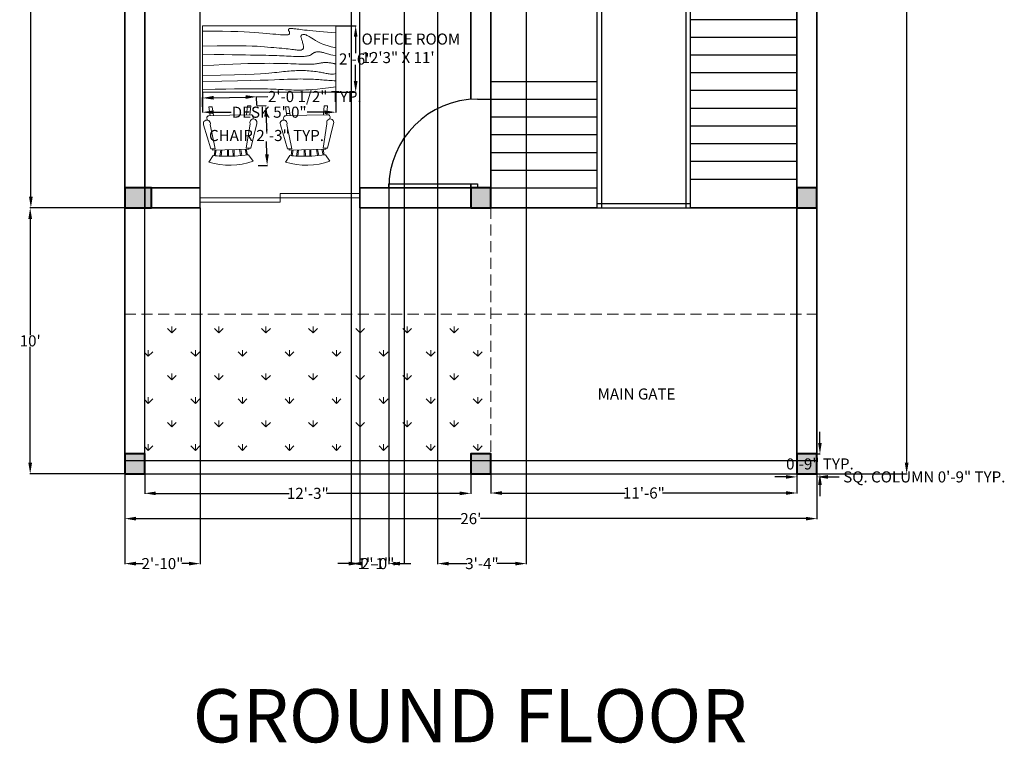
# Model space of a CAD drawing. Units: inches. Extents: x -54 to 881, y -122 to 681.
# Tile 1 of 6: x -47 to 396, y -121 to 205. Entities that reach past the tile are written whole.
import ezdxf

# ---------------------------------------------------------------- set-up
doc = ezdxf.new("R2010")
doc.units = ezdxf.units.IN
doc.header["$MEASUREMENT"] = 0
doc.linetypes.add('DASHED', pattern=[0.75, 0.5, -0.25])
for name, color, linetype, lineweight in [('A-ANNO-DIMS', 2, 'Continuous', 18), ('A-ANNO-TITL', 7, 'Continuous', 35), ('A-DOOR', 3, 'Continuous', 25), ('A-FLOR-OVHD', 8, 'DASHED', 18), ('A-FLOR-STRS', 7, 'Continuous', 25), ('A-FURN', 8, 'Continuous', 18), ('A-GLAZ', 4, 'Continuous', 20), ('A-WALL', 7, 'Continuous', 35), ('A-WALL-SITE', 7, 'Continuous', 30), ('L-PLNT-PATT', 9, 'Continuous', 13)]:
    doc.layers.add(name, color=color, linetype=linetype, lineweight=lineweight)
for name, color, linetype, lineweight, true_color in [('A-ANNO-TEXT', 217, 'Continuous', 18, 0x93278f), ('A-AREA-IDEN', 217, 'Continuous', 18, 0x93278f), ('A-COLS', 240, 'Continuous', 40, 0xed1f24)]:
    doc.layers.add(name, color=color, linetype=linetype, lineweight=lineweight, true_color=true_color)
doc.styles.get("Standard").update_dxf_attribs({"font": 'arial.ttf'})
doc.dimstyles.get("Standard").update_dxf_attribs({"dimtxt": 5, "dimasz": 5, "dimexe": 0.18, "dimexo": 0.0625, "dimgap": 0.09, "dimtad": 0, "dimtih": 1, "dimtoh": 1, "dimdec": 0, "dimzin": 0, "dimdsep": 46, "dimlunit": 3, "dimtxsty": 'Standard', "dimcen": 0.09, "dimadec": 0, "dimazin": 0, "dimtfac": 1, "dimtdec": 0, "dimtofl": 0, "dimtmove": 0, "dimatfit": 3, "dimfxl": 1, "dimtolj": 1, "dimtzin": 0, "dimarcsym": 0})

# ---------------------------------------------------------------- blocks, each defined once
blk = doc.blocks.new('*D2')
at = {"layer": 'A-ANNO-DIMS', "color": 0, "lineweight": -2, "transparency": 16777216}
for p, q in [((-0.06, 624), (-42.51, 624)), ((-42.33, 619), (-42.33, 374.6)), ((-42.33, 125), (-42.33, 369.4)), ((-0.06, 120), (-42.51, 120))]:
    blk.add_line(p, q, dxfattribs=at)
at = {"layer": 'A-ANNO-DIMS', "color": 0, "transparency": 16777216}
for points in [[(-43.17, 619), (-41.5, 619), (-42.33, 624)], [(-43.17, 125), (-41.5, 125), (-42.33, 120)]]:
    blk.add_solid(points, dxfattribs=at)
at = {"layer": 'Defpoints', "color": 0, "transparency": 16777216}
for p in [(0, 624), (-42.33, 120), (0, 120)]:
    blk.add_point(p, dxfattribs=at)
at = {"layer": 'A-ANNO-DIMS', "color": 0, "transparency": 16777216, "insert": (-42.33, 372), "char_height": 5, "attachment_point": 5}
blk.add_mtext("\\A1;42'", dxfattribs=at)
blk = doc.blocks.new('Table - Rectangular Woodgrain 60 x 30 in.')
for p, q in [((0, 0), (0, -30)), ((60, 0), (0, 0)), ((60, -30), (60, 0)), ((0, -30), (60, -30))]:
    blk.add_line(p, q)
for points in [[(0, -2.4), (4.8155, -2.418), (9.0302, -2.4688), (12.709, -2.5477), (15.9167, -2.65), (18.7181, -2.7711), (21.1781, -2.9063), (23.3616, -3.0508), (25.3333, -3.2), (27.1477, -3.3495), (28.8172, -3.4958), (30.3437, -3.636), (31.7291, -3.7667), (32.9756, -3.8849), (34.0849, -3.9875), (35.059, -4.0714), (35.9, -4.1334), (36.6114, -4.1711), (37.2041, -4.1854), (37.6906, -4.1779), (38.0833, -4.15), (38.3948, -4.1034), (38.6375, -4.0396), (38.8239, -3.9602), (38.9666, -3.8667), (39.0764, -3.7608), (39.1573, -3.6448), (39.2116, -3.521), (39.2416, -3.3917), (39.2498, -3.2593), (39.2385, -3.1261), (39.21, -2.9944), (39.1666, -2.8667), (39.111, -2.7447), (39.0468, -2.6281), (38.978, -2.5163), (38.9083, -2.4083), (38.8418, -2.3035), (38.7823, -2.201), (38.7337, -2.1001), (38.7, -2), (38.6844, -1.9003), (38.6875, -1.8021), (38.7094, -1.707), (38.75, -1.6167), (38.8094, -1.5326), (38.8875, -1.4563), (38.9844, -1.3893), (39.1, -1.3333), (39.2351, -1.2896), (39.3937, -1.2583), (39.5804, -1.2396), (39.8, -1.2333), (40.057, -1.2396), (40.3562, -1.2583), (40.7023, -1.2896), (41.1, -1.3333), (41.5547, -1.3895), (42.0755, -1.4573), (42.6721, -1.5361), (43.3542, -1.625), (44.1316, -1.7233), (45.014, -1.8302), (46.0114, -1.9449), (47.1333, -2.0667), (48.3862, -2.1947), (49.7625, -2.3281), (51.2513, -2.4663), (52.8416, -2.6083), (54.5226, -2.7535), (56.2833, -2.9011), (58.1127, -3.0501), (60, -3.2)], [(0, -9.2), (6.5759, -9.0858), (11.9385, -9.0365), (16.2527, -9.0418), (19.6833, -9.0917), (22.3952, -9.1759), (24.5531, -9.2844), (26.322, -9.4069), (27.8666, -9.5333), (29.3241, -9.6553), (30.7203, -9.7719), (32.0532, -9.8837), (33.3208, -9.9917), (34.5213, -10.0965), (35.6526, -10.199), (36.7128, -10.2999), (37.7, -10.4), (38.6129, -10.4996), (39.4531, -10.5969), (40.223, -10.6895), (40.925, -10.775), (41.5613, -10.8512), (42.1344, -10.9156), (42.6465, -10.966), (43.1, -11), (43.4976, -11.0158), (43.8437, -11.0136), (44.143, -10.9942), (44.4, -10.9583), (44.6195, -10.9069), (44.8062, -10.8406), (44.9648, -10.7603), (45.1, -10.6667), (45.2155, -10.5598), (45.3114, -10.4365), (45.3871, -10.2929), (45.4416, -10.125), (45.4743, -9.929), (45.4844, -9.7011), (45.4709, -9.4371), (45.4333, -9.1333), (45.3716, -8.7883), (45.2896, -8.4104), (45.1919, -8.0107), (45.0833, -7.6), (44.9685, -7.1893), (44.8521, -6.7896), (44.7388, -6.4117), (44.6333, -6.0667), (44.54, -5.7628), (44.4614, -5.4979), (44.4001, -5.2675), (44.3583, -5.0667), (44.3384, -4.8909), (44.3427, -4.7354), (44.3736, -4.5956), (44.4333, -4.4667), (44.5236, -4.3453), (44.6427, -4.2333), (44.7884, -4.1339), (44.9583, -4.05), (45.1501, -3.9849), (45.3614, -3.9417), (45.59, -3.9234), (45.8333, -3.9333), (46.0915, -3.9749), (46.3734, -4.0531), (46.6906, -4.1736), (47.0542, -4.3417), (47.4756, -4.5629), (47.9661, -4.8427), (48.5372, -5.1866), (49.2, -5.6), (49.9676, -6.0844), (50.8594, -6.625), (51.8965, -7.2031), (53.1, -7.8), (54.491, -8.3969), (56.0906, -8.975), (57.9199, -9.5156), (60, -10)], [(0, -12.8), (5.1847, -12.9322), (9.6213, -13.0323), (13.3963, -13.1059), (16.5958, -13.1583), (19.3063, -13.1952), (21.614, -13.2219), (23.6054, -13.2439), (25.3666, -13.2667), (26.9728, -13.2947), (28.4531, -13.3281), (29.8256, -13.3663), (31.1083, -13.4083), (32.3191, -13.4535), (33.476, -13.501), (34.597, -13.5501), (35.7, -13.6), (36.7984, -13.6497), (37.8875, -13.6979), (38.9578, -13.743), (40, -13.7833), (41.0047, -13.8174), (41.9625, -13.8438), (42.864, -13.8607), (43.7, -13.8667), (44.4631, -13.8604), (45.1552, -13.8417), (45.7801, -13.8104), (46.3416, -13.7667), (46.8439, -13.7104), (47.2906, -13.6417), (47.6858, -13.5604), (48.0333, -13.4667), (48.3375, -13.3608), (48.6042, -13.2448), (48.8396, -13.121), (49.05, -12.9917), (49.2417, -12.8593), (49.4208, -12.7261), (49.5937, -12.5944), (49.7667, -12.4667), (49.9452, -12.3451), (50.1323, -12.2313), (50.3303, -12.1268), (50.5416, -12.0333), (50.7686, -11.9524), (51.0135, -11.8854), (51.2788, -11.8341), (51.5666, -11.8), (51.8785, -11.7843), (52.2116, -11.7865), (52.562, -11.8059), (52.926, -11.8417), (53.2998, -11.8931), (53.6795, -11.9594), (54.0614, -12.0397), (54.4416, -12.1333), (54.8223, -12.2401), (55.2293, -12.3625), (55.6942, -12.5037), (56.2489, -12.6667), (56.9251, -12.8547), (57.7545, -13.0708), (58.7689, -13.3182), (60, -13.6)], [(0, -18), (5.124, -17.7273), (9.6609, -17.5057), (13.6705, -17.3303), (17.2125, -17.1958), (20.3467, -17.0973), (23.1328, -17.0297), (25.6307, -16.9878), (27.9, -16.9667), (29.9928, -16.9617), (31.9302, -16.9703), (33.7254, -16.9907), (35.3917, -17.0208), (36.9423, -17.0588), (38.3906, -17.1026), (39.7499, -17.1503), (41.0333, -17.2), (42.2519, -17.2496), (43.4073, -17.2969), (44.4986, -17.3395), (45.525, -17.375), (46.4858, -17.4012), (47.3802, -17.4156), (48.2074, -17.416), (48.9667, -17.4), (49.6583, -17.3662), (50.2872, -17.3167), (50.8595, -17.2547), (51.3812, -17.1833), (51.8584, -17.1057), (52.2971, -17.025), (52.7034, -16.9443), (53.0833, -16.8667), (53.443, -16.7951), (53.789, -16.7313), (54.128, -16.6768), (54.4666, -16.6334), (54.8115, -16.6024), (55.1693, -16.5854), (55.5465, -16.5841), (55.95, -16.6), (56.3828, -16.6337), (56.8346, -16.6823), (57.2915, -16.7418), (57.7396, -16.8084), (58.165, -16.878), (58.5539, -16.9469), (58.8924, -17.0111), (59.1666, -17.0667), (59.3679, -17.1107), (59.5078, -17.1438), (59.6032, -17.1675), (59.6708, -17.1833), (59.7275, -17.193), (59.7901, -17.1979), (59.8753, -17.1998), (60, -17.2)], [(0, -22.4), (8.0098, -22.2501), (14.4094, -22.1011), (19.4168, -21.9535), (23.25, -21.8083), (26.1269, -21.6663), (28.2656, -21.5281), (29.884, -21.3947), (31.2, -21.2667), (32.3967, -21.1448), (33.5172, -21.0292), (34.5697, -20.9198), (35.5625, -20.8167), (36.5037, -20.7198), (37.4015, -20.6292), (38.2642, -20.5448), (39.1, -20.4667), (39.9164, -20.3951), (40.7187, -20.3313), (41.5117, -20.2768), (42.3, -20.2333), (43.0883, -20.2024), (43.8812, -20.1854), (44.6836, -20.1841), (45.5, -20.2), (46.3328, -20.234), (47.1747, -20.2844), (48.0163, -20.3488), (48.8479, -20.425), (49.66, -20.5106), (50.4429, -20.6031), (51.1872, -20.7004), (51.8833, -20.8), (52.5246, -20.8999), (53.1166, -20.9995), (53.6681, -21.0983), (54.1875, -21.1958), (54.6834, -21.2919), (55.1646, -21.3859), (55.6394, -21.4777), (56.1167, -21.5667), (56.6028, -21.6515), (57.0961, -21.7266), (57.5929, -21.7852), (58.0896, -21.8208), (58.5823, -21.8268), (59.0674, -21.7964), (59.5412, -21.723), (60, -21.6)], [(0, -25.2), (8.6355, -25.0504), (15.7026, -24.9031), (21.4049, -24.7606), (25.9458, -24.625), (29.529, -24.4988), (32.3578, -24.3844), (34.6359, -24.284), (36.5667, -24.2), (38.3213, -24.1341), (39.9417, -24.0854), (41.437, -24.0523), (42.8167, -24.0333), (44.0901, -24.0268), (45.2667, -24.0313), (46.3557, -24.0451), (47.3667, -24.0667), (48.309, -24.0947), (49.1928, -24.1287), (50.0284, -24.168), (50.826, -24.2125), (51.5959, -24.2617), (52.3483, -24.3151), (53.0935, -24.3725), (53.8417, -24.4334), (54.6009, -24.497), (55.3699, -24.561), (56.1454, -24.6226), (56.9239, -24.6792), (57.7021, -24.7279), (58.4764, -24.7662), (59.2435, -24.7911), (60, -24.8)], [(0, -28.8), (5.6867, -28.6681), (10.45, -28.5698), (14.407, -28.5012), (17.675, -28.4584), (20.3711, -28.4374), (22.6125, -28.4344), (24.5164, -28.4455), (26.2, -28.4667), (27.762, -28.4947), (29.2276, -28.5281), (30.6033, -28.5663), (31.8958, -28.6084), (33.1118, -28.6535), (34.2578, -28.7011), (35.3405, -28.7501), (36.3666, -28.8), (37.3443, -28.8497), (38.288, -28.8974), (39.2137, -28.9412), (40.1375, -28.9792), (41.0753, -29.0093), (42.0432, -29.0297), (43.0572, -29.0384), (44.1333, -29.0333), (45.2936, -29.0114), (46.5843, -28.9641), (48.0579, -28.8816), (49.7666, -28.7542), (51.7629, -28.5721), (54.0989, -28.3255), (56.8272, -28.0048), (60, -27.6)]]:
    blk.add_lwpolyline(points)
blk = doc.blocks.new('Chair - Rocking')
for p, q in [((-8, -4.5), (-10, -1.5)), ((-6.5, -7), (-7.02225, -4.43)), ((-4.5, -7), (-4.96674, -4.19951)), ((-4, -7), (-4.40532, -4.16272)), ((-1.5, -4.05012), (-1.5, -7)), ((-1, -7), (-1, -4.05012)), ((1, -7), (1, -4.04655)), ((1.5, -4.05012), (1.5, -7)), ((4, -7), (4.40187, -4.18694)), ((4.5, -7), (4.96761, -4.19437)), ((6.5, -7), (7, -4.4057)), ((8, -4.5), (10, -1.5)), ((-9, -7.5), (-12, -18.49999)), ((-7, -7.5), (-9, -7.5)), ((-9, -18.49999), (-7, -7.5)), ((-8.23428, -6.99939), (-8.3093, -7.47958)), ((-8.23041, -7), (8.23915, -7)), ((-7.5, -4.5), (-7, -7)), ((7.5, -4.5), (7, -7)), ((7, -7.5), (9, -7.5)), ((9, -18.49999), (7, -7.5)), ((8.31071, -7.48854), (8.23449, -7.00073)), ((9, -7.5), (12, -18.49999)), ((-10.36644, -20.64523), (-10.5, -21.49999)), ((10.5, -21.49999), (10.3575, -20.58798)), ((-9, -22.49999), (-9.5, -26.49999)), ((0, -22.49999), (-9.5, -22.49999)), ((-9.5, -26.49999), (-8, -26.49999)), ((-8, -26.49999), (-7.5, -22.49999)), ((0, -22.49999), (9.5, -22.49999)), ((8, -26.49999), (7.5, -22.49999)), ((9.5, -26.49999), (8, -26.49999)), ((9, -22.49999), (9.5, -26.49999))]:
    blk.add_line(p, q)
for centre, radius, start, end in [((0, -34.08333), 34.08333, 72.93847, 107.0615), ((0, -68.25004), 64.25, 93.92211, 97.15267), ((0, -68.25004), 64.25, 82.84733, 93.92211), ((-10.5, -18.99999), 1.58114, 161.5651, 18.43495), ((-9.5, -21.49999), 1, 180, 270), ((10.5, -18.99999), 1.58114, 161.5651, 18.43495), ((9.5, -21.49999), 1, 270, 0)]:
    blk.add_arc(centre, radius, start, end)
blk = doc.blocks.new('*U12')
for p, q in [((0, 0), (0, -6)), ((40, 0), (40, -6))]:
    blk.add_line(p, q)
blk.add_lwpolyline([(0, 0), (0, 40), (1.75, 40), (1.75, 0)], close=True)
blk.add_arc((0, 0), 40, 0, 90)
blk = doc.blocks.new('*D17')
at = {"layer": 'A-ANNO-DIMS', "color": 0, "lineweight": -2, "transparency": 16777216}
for p, q in [((-0.06, 120), (-42.81, 120)), ((-42.63, 115), (-42.63, 62.64)), ((-42.63, 5), (-42.63, 57.36)), ((-0.06, 0), (-42.81, 0))]:
    blk.add_line(p, q, dxfattribs=at)
at = {"layer": 'A-ANNO-DIMS', "color": 0, "transparency": 16777216}
for points in [[(-43.46, 115), (-41.8, 115), (-42.63, 120)], [(-43.46, 5), (-41.8, 5), (-42.63, 0)]]:
    blk.add_solid(points, dxfattribs=at)
at = {"layer": 'Defpoints', "color": 0, "transparency": 16777216}
for p in [(0, 120), (0, 0), (-42.63, 0)]:
    blk.add_point(p, dxfattribs=at)
at = {"layer": 'A-ANNO-DIMS', "color": 0, "transparency": 16777216, "insert": (-42.63, 60), "char_height": 5, "attachment_point": 5}
blk.add_mtext("\\A1;10'", dxfattribs=at)
blk = doc.blocks.new('*D18')
at = {"layer": 'A-ANNO-DIMS', "color": 0, "lineweight": -2, "transparency": 16777216}
for p, q in [((9, -0.06), (9, -8.94)), ((156, -0.06), (156, -8.94)), ((14, -8.76), (74.06, -8.76)), ((151, -8.76), (90.94, -8.76))]:
    blk.add_line(p, q, dxfattribs=at)
at = {"layer": 'A-ANNO-DIMS', "color": 0, "transparency": 16777216}
for points in [[(14, -7.93), (14, -9.59), (9, -8.76)], [(151, -7.93), (151, -9.59), (156, -8.76)]]:
    blk.add_solid(points, dxfattribs=at)
at = {"layer": 'Defpoints', "color": 0, "transparency": 16777216}
for p in [(9, 0), (156, 0), (156, -8.76)]:
    blk.add_point(p, dxfattribs=at)
at = {"layer": 'A-ANNO-DIMS', "color": 0, "transparency": 16777216, "insert": (82.5, -8.76), "char_height": 5, "attachment_point": 5}
blk.add_mtext('\\A1;12\'-3"', dxfattribs=at)
blk = doc.blocks.new('*D19')
at = {"layer": 'A-ANNO-DIMS', "color": 0, "lineweight": -2, "transparency": 16777216}
for p, q in [((165, -0.06), (165, -8.79)), ((303, -0.06), (303, -8.79)), ((170, -8.61), (225.56, -8.61)), ((298, -8.61), (242.44, -8.61))]:
    blk.add_line(p, q, dxfattribs=at)
at = {"layer": 'A-ANNO-DIMS', "color": 0, "transparency": 16777216}
for points in [[(170, -7.78), (170, -9.45), (165, -8.61)], [(298, -7.78), (298, -9.45), (303, -8.61)]]:
    blk.add_solid(points, dxfattribs=at)
at = {"layer": 'Defpoints', "color": 0, "transparency": 16777216}
for p in [(165, 0), (303, 0), (303, -8.61)]:
    blk.add_point(p, dxfattribs=at)
at = {"layer": 'A-ANNO-DIMS', "color": 0, "transparency": 16777216, "insert": (234, -8.61), "char_height": 5, "attachment_point": 5}
blk.add_mtext('\\A1;11\'-6"', dxfattribs=at)
blk = doc.blocks.new('*D20')
at = {"layer": 'A-ANNO-DIMS', "color": 0, "lineweight": -2, "transparency": 16777216}
for p, q in [((0, -0.06), (0, -20.34)), ((312, -0.06), (312, -20.34)), ((5, -20.16), (151.62, -20.16)), ((307, -20.16), (160.38, -20.16))]:
    blk.add_line(p, q, dxfattribs=at)
at = {"layer": 'A-ANNO-DIMS', "color": 0, "transparency": 16777216}
for points in [[(5, -19.33), (5, -20.99), (0, -20.16)], [(307, -19.33), (307, -20.99), (312, -20.16)]]:
    blk.add_solid(points, dxfattribs=at)
at = {"layer": 'Defpoints', "color": 0, "transparency": 16777216}
for p in [(0, 0), (312, 0), (312, -20.16)]:
    blk.add_point(p, dxfattribs=at)
at = {"layer": 'A-ANNO-DIMS', "color": 0, "transparency": 16777216, "insert": (156, -20.16), "char_height": 5, "attachment_point": 5}
blk.add_mtext("\\A1;26'", dxfattribs=at)
blk = doc.blocks.new('STAIR-RETURN-FLIGHT')
for p, q in [((48, 93), (48, 141)), ((56.4, 93), (56.4, 141)), ((64.8, 93), (64.8, 141)), ((73.2, 93), (73.2, 141)), ((81.6, 93), (81.6, 141)), ((90, 93), (90, 141)), ((48, 0), (48, 93)), ((48, 93), (90, 93)), ((48, 91), (90, 91)), ((50, 0), (50, 93)), ((88, 0), (88, 93)), ((90, 0), (90, 93)), ((90, 93), (138, 93)), ((90, 85), (138, 85)), ((90, 77), (138, 77)), ((90, 69), (138, 69)), ((90, 61), (138, 61)), ((0, 57), (48, 57)), ((0, 49), (48, 49)), ((90, 53), (138, 53)), ((90, 45), (138, 45)), ((0, 41), (48, 41)), ((90, 37), (138, 37)), ((0, 33), (48, 33)), ((90, 29), (138, 29)), ((0, 25), (48, 25)), ((90, 21), (138, 21)), ((0, 17), (48, 17)), ((0, 9), (48, 9)), ((90, 13), (138, 13)), ((48, 2), (90, 2)), ((48, 0), (90, 0))]:
    blk.add_line(p, q)
blk = doc.blocks.new('COL-9X12')
h = blk.add_hatch(color=256)
h.dxf.hatch_style = 1
h.paths.add_polyline_path([(9, 12), (0, 12), (0, 0), (9, 0)])
blk.add_lwpolyline([(0, 0), (9, 0), (9, 12), (0, 12)], close=True)
blk = doc.blocks.new('COL-9X9')
h = blk.add_hatch(color=256)
h.dxf.hatch_style = 1
h.paths.add_polyline_path([(9, 9), (0, 9), (0, 0), (9, 0)])
blk.add_lwpolyline([(0, 0), (9, 0), (9, 9), (0, 9)], close=True)
blk = doc.blocks.new('*D38')
at = {"layer": 'A-ANNO-DIMS', "color": 0, "lineweight": -2, "transparency": 16777216}
for p, q in [((298, -1.35), (293, -1.35)), ((303, -0.06), (303, -1.53)), ((312, -0.06), (312, -1.53)), ((317, -1.35), (322, -1.35))]:
    blk.add_line(p, q, dxfattribs=at)
at = {"layer": 'A-ANNO-DIMS', "color": 0, "transparency": 16777216}
for points in [[(298, -0.52), (298, -2.18), (303, -1.35)], [(317, -0.52), (317, -2.18), (312, -1.35)]]:
    blk.add_solid(points, dxfattribs=at)
at = {"layer": 'Defpoints', "color": 0, "transparency": 16777216}
for p in [(303, 0), (312, 0), (312, -1.35)]:
    blk.add_point(p, dxfattribs=at)
at = {"layer": 'A-ANNO-DIMS', "color": 0, "transparency": 16777216, "insert": (360.41, -1.35), "char_height": 5, "attachment_point": 5}
blk.add_mtext('\\A1;SQ. COLUMN 0\'-9" TYP.', dxfattribs=at)
blk = doc.blocks.new('*D39')
at = {"layer": 'A-ANNO-DIMS', "color": 0, "lineweight": -2, "transparency": 16777216}
for p, q in [((313.35, 14), (313.35, 19)), ((312.06, 9), (313.53, 9)), ((312.06, 0), (313.53, 0)), ((313.35, -5), (313.35, -10))]:
    blk.add_line(p, q, dxfattribs=at)
at = {"layer": 'A-ANNO-DIMS', "color": 0, "transparency": 16777216}
for points in [[(312.52, 14), (314.18, 14), (313.35, 9)], [(312.52, -5), (314.18, -5), (313.35, 0)]]:
    blk.add_solid(points, dxfattribs=at)
at = {"layer": 'Defpoints', "color": 0, "transparency": 16777216}
for p in [(312, 9), (313.35, 9), (312, 0)]:
    blk.add_point(p, dxfattribs=at)
at = {"layer": 'A-ANNO-DIMS', "color": 0, "transparency": 16777216, "insert": (313.35, 4.5), "char_height": 5, "attachment_point": 5}
blk.add_mtext('\\A1;0\'-9" TYP.', dxfattribs=at)
blk = doc.blocks.new('*D46')
at = {"layer": 'A-ANNO-DIMS', "color": 0, "lineweight": -2, "transparency": 16777216}
for p, q in [((59.61, 166.03), (63.77, 166.12)), ((63.7, 161.12), (63.83, 155.3)), ((64.08, 144.12), (63.95, 149.94)), ((60.2, 139.04), (64.37, 139.13))]:
    blk.add_line(p, q, dxfattribs=at)
at = {"layer": 'A-ANNO-DIMS', "color": 0, "transparency": 16777216}
for points in [[(64.54, 161.14), (62.87, 161.1), (63.59, 166.12)], [(64.91, 144.14), (63.25, 144.11), (64.19, 139.12)]]:
    blk.add_solid(points, dxfattribs=at)
at = {"layer": 'Defpoints', "color": 0, "transparency": 16777216}
for p in [(59.54, 166.03), (60.14, 139.04), (64.19, 139.12)]:
    blk.add_point(p, dxfattribs=at)
at = {"layer": 'A-ANNO-DIMS', "color": 0, "transparency": 16777216, "insert": (63.89, 152.62), "char_height": 5, "attachment_point": 5}
blk.add_mtext('\\A1;CHAIR 2\'-3" TYP.', dxfattribs=at)
blk = doc.blocks.new('*D47')
at = {"layer": 'A-ANNO-DIMS', "color": 0, "lineweight": -2, "transparency": 16777216}
for p, q in [((35.11, 165.55), (35.02, 169.72)), ((40.02, 169.65), (54.46, 169.97)), ((59.54, 166.09), (59.45, 170.26)), ((59.45, 170.08), (64.45, 170.19))]:
    blk.add_line(p, q, dxfattribs=at)
at = {"layer": 'A-ANNO-DIMS', "color": 0, "transparency": 16777216}
for points in [[(40.01, 170.48), (40.04, 168.81), (35.02, 169.54)], [(54.44, 170.8), (54.47, 169.13), (59.45, 170.08)]]:
    blk.add_solid(points, dxfattribs=at)
at = {"layer": 'Defpoints', "color": 0, "transparency": 16777216}
for p in [(59.45, 170.08), (35.11, 165.49), (59.54, 166.03)]:
    blk.add_point(p, dxfattribs=at)
at = {"layer": 'A-ANNO-DIMS', "color": 0, "transparency": 16777216, "insert": (85.65, 170.19), "char_height": 5, "attachment_point": 5}
blk.add_mtext('\\A1;2\'-0 1/2" TYP.', dxfattribs=at)
blk = doc.blocks.new('*D48')
at = {"layer": 'A-ANNO-DIMS', "color": 0, "lineweight": -2, "transparency": 16777216}
for p, q in [((35.08, 172.07), (35.08, 162.95)), ((95.08, 172.07), (95.08, 162.95)), ((40.08, 163.13), (47.98, 163.13)), ((90.08, 163.13), (82.17, 163.13))]:
    blk.add_line(p, q, dxfattribs=at)
at = {"layer": 'A-ANNO-DIMS', "color": 0, "transparency": 16777216}
for points in [[(40.08, 163.96), (40.08, 162.29), (35.08, 163.13)], [(90.08, 163.96), (90.08, 162.29), (95.08, 163.13)]]:
    blk.add_solid(points, dxfattribs=at)
at = {"layer": 'Defpoints', "color": 0, "transparency": 16777216}
for p in [(35.08, 172.13), (95.08, 172.13), (95.08, 163.13)]:
    blk.add_point(p, dxfattribs=at)
at = {"layer": 'A-ANNO-DIMS', "color": 0, "transparency": 16777216, "insert": (65.08, 163.13), "char_height": 5, "attachment_point": 5}
blk.add_mtext('\\A1;DESK 5\'-0"', dxfattribs=at)
blk = doc.blocks.new('*D49')
at = {"layer": 'A-ANNO-DIMS', "color": 0, "lineweight": -2, "transparency": 16777216}
for p, q in [((95.14, 202.13), (104.26, 202.13)), ((104.08, 197.13), (104.08, 189.77)), ((104.08, 177.13), (104.08, 184.49)), ((95.14, 172.13), (104.26, 172.13))]:
    blk.add_line(p, q, dxfattribs=at)
at = {"layer": 'A-ANNO-DIMS', "color": 0, "transparency": 16777216}
for points in [[(103.24, 197.13), (104.91, 197.13), (104.08, 202.13)], [(103.24, 177.13), (104.91, 177.13), (104.08, 172.13)]]:
    blk.add_solid(points, dxfattribs=at)
at = {"layer": 'Defpoints', "color": 0, "transparency": 16777216}
for p in [(95.08, 202.13), (104.08, 202.13), (95.08, 172.13)]:
    blk.add_point(p, dxfattribs=at)
at = {"layer": 'A-ANNO-DIMS', "color": 0, "transparency": 16777216, "insert": (104.08, 187.13), "char_height": 5, "attachment_point": 5}
blk.add_mtext('\\A1;2\'-6"', dxfattribs=at)
blk = doc.blocks.new('*D74')
at = {"layer": 'A-ANNO-DIMS', "color": 0, "lineweight": -2, "transparency": 16777216}
for p, q in [((312.06, 624), (352.63, 624)), ((352.45, 619), (352.45, 314.64)), ((352.45, 5), (352.45, 309.36)), ((312.06, 0), (352.63, 0))]:
    blk.add_line(p, q, dxfattribs=at)
at = {"layer": 'A-ANNO-DIMS', "color": 0, "transparency": 16777216}
for points in [[(351.62, 619), (353.28, 619), (352.45, 624)], [(351.62, 5), (353.28, 5), (352.45, 0)]]:
    blk.add_solid(points, dxfattribs=at)
at = {"layer": 'Defpoints', "color": 0, "transparency": 16777216}
for p in [(312, 624), (352.45, 624), (312, 0)]:
    blk.add_point(p, dxfattribs=at)
at = {"layer": 'A-ANNO-DIMS', "color": 0, "transparency": 16777216, "insert": (352.45, 312), "char_height": 5, "attachment_point": 5}
blk.add_mtext('\\A1;52\'-0"', dxfattribs=at)
blk = doc.blocks.new('*D76')
at = {"layer": 'A-ANNO-DIMS', "color": 0, "lineweight": -2, "transparency": 16777216}
for p, q in [((102, 545.94), (102, -40.63)), ((126, 548.94), (126, -40.63)), ((107, -40.45), (107.22, -40.45)), ((121, -40.45), (120.78, -40.45))]:
    blk.add_line(p, q, dxfattribs=at)
at = {"layer": 'A-ANNO-DIMS', "color": 0, "transparency": 16777216}
for points in [[(107, -39.62), (107, -41.28), (102, -40.45)], [(121, -39.62), (121, -41.28), (126, -40.45)]]:
    blk.add_solid(points, dxfattribs=at)
at = {"layer": 'Defpoints', "color": 0, "transparency": 16777216}
for p in [(102, 546), (126, 549), (126, -40.45)]:
    blk.add_point(p, dxfattribs=at)
at = {"layer": 'A-ANNO-DIMS', "color": 0, "transparency": 16777216, "insert": (114, -40.45), "char_height": 5, "attachment_point": 5}
blk.add_mtext('\\A1;2\'-0"', dxfattribs=at)
blk = doc.blocks.new('*D77')
at = {"layer": 'A-ANNO-DIMS', "color": 0, "lineweight": -2, "transparency": 16777216}
for p, q in [((141, 461.94), (141, -40.63)), ((181, 461.94), (181, -40.63)), ((146, -40.45), (154.27, -40.45)), ((176, -40.45), (167.73, -40.45))]:
    blk.add_line(p, q, dxfattribs=at)
at = {"layer": 'A-ANNO-DIMS', "color": 0, "transparency": 16777216}
for points in [[(146, -39.62), (146, -41.28), (141, -40.45)], [(176, -39.62), (176, -41.28), (181, -40.45)]]:
    blk.add_solid(points, dxfattribs=at)
at = {"layer": 'Defpoints', "color": 0, "transparency": 16777216}
for p in [(141, 462), (181, 462), (181, -40.45)]:
    blk.add_point(p, dxfattribs=at)
at = {"layer": 'A-ANNO-DIMS', "color": 0, "transparency": 16777216, "insert": (161, -40.45), "char_height": 5, "attachment_point": 5}
blk.add_mtext('\\A1;3\'-4"', dxfattribs=at)
blk = doc.blocks.new('*D84')
at = {"layer": 'A-ANNO-DIMS', "color": 0, "lineweight": -2, "transparency": 16777216}
for p, q in [((0, 119.94), (0, -40.63)), ((33.99, 119.94), (33.99, -40.63)), ((5, -40.45), (8.27, -40.45)), ((28.99, -40.45), (25.71, -40.45))]:
    blk.add_line(p, q, dxfattribs=at)
at = {"layer": 'A-ANNO-DIMS', "color": 0, "transparency": 16777216}
for points in [[(5, -39.62), (5, -41.28), (0, -40.45)], [(28.99, -39.62), (28.99, -41.28), (33.99, -40.45)]]:
    blk.add_solid(points, dxfattribs=at)
at = {"layer": 'Defpoints', "color": 0, "transparency": 16777216}
for p in [(0, 120), (33.99, 120), (33.99, -40.45)]:
    blk.add_point(p, dxfattribs=at)
at = {"layer": 'A-ANNO-DIMS', "color": 0, "transparency": 16777216, "insert": (16.99, -40.45), "char_height": 5, "attachment_point": 5}
blk.add_mtext('\\A1;2\'-10"', dxfattribs=at)
blk = doc.blocks.new('*D85')
at = {"layer": 'A-ANNO-DIMS', "color": 0, "lineweight": -2, "transparency": 16777216}
for p, q in [((33.99, 120.06), (33.99, 664.63)), ((38.99, 664.45), (63.24, 664.45)), ((100.99, 664.45), (76.73, 664.45)), ((105.99, 120.06), (105.99, 664.63))]:
    blk.add_line(p, q, dxfattribs=at)
at = {"layer": 'A-ANNO-DIMS', "color": 0, "transparency": 16777216}
for points in [[(38.99, 665.28), (38.99, 663.62), (33.99, 664.45)], [(100.99, 665.28), (100.99, 663.62), (105.99, 664.45)]]:
    blk.add_solid(points, dxfattribs=at)
at = {"layer": 'Defpoints', "color": 0, "transparency": 16777216}
for p in [(105.99, 664.45), (33.99, 120), (105.99, 120)]:
    blk.add_point(p, dxfattribs=at)
at = {"layer": 'A-ANNO-DIMS', "color": 0, "transparency": 16777216, "insert": (69.99, 664.45), "char_height": 5, "attachment_point": 5}
blk.add_mtext('\\A1;6\'-0"', dxfattribs=at)
blk = doc.blocks.new('*D86')
at = {"layer": 'A-ANNO-DIMS', "color": 0, "lineweight": -2, "transparency": 16777216}
for p, q in [((105.99, 128.94), (105.99, -40.63)), ((119, 128.94), (119, -40.63)), ((100.99, -40.45), (95.99, -40.45)), ((124, -40.45), (129, -40.45))]:
    blk.add_line(p, q, dxfattribs=at)
at = {"layer": 'A-ANNO-DIMS', "color": 0, "transparency": 16777216}
for points in [[(100.99, -39.62), (100.99, -41.28), (105.99, -40.45)], [(124, -39.62), (124, -41.28), (119, -40.45)]]:
    blk.add_solid(points, dxfattribs=at)
at = {"layer": 'Defpoints', "color": 0, "transparency": 16777216}
for p in [(105.99, 129), (119, 129), (119, -40.45)]:
    blk.add_point(p, dxfattribs=at)
at = {"layer": 'A-ANNO-DIMS', "color": 0, "transparency": 16777216, "insert": (112.49, -40.45), "char_height": 5, "attachment_point": 5}
blk.add_mtext('\\A1;1\'-1"', dxfattribs=at)
blk = doc.blocks.new('*D89')
at = {"layer": 'A-ANNO-DIMS', "color": 0, "lineweight": -2, "transparency": 16777216}
for p, q in [((165, 120.06), (165, 664.63)), ((170, 664.45), (182.16, 664.45)), ((208, 664.45), (195.84, 664.45)), ((213, 120.06), (213, 664.63))]:
    blk.add_line(p, q, dxfattribs=at)
at = {"layer": 'A-ANNO-DIMS', "color": 0, "transparency": 16777216}
for points in [[(170, 665.28), (170, 663.62), (165, 664.45)], [(208, 665.28), (208, 663.62), (213, 664.45)]]:
    blk.add_solid(points, dxfattribs=at)
at = {"layer": 'Defpoints', "color": 0, "transparency": 16777216}
for p in [(213, 664.45), (165, 120), (213, 120)]:
    blk.add_point(p, dxfattribs=at)
at = {"layer": 'A-ANNO-DIMS', "color": 0, "transparency": 16777216, "insert": (189, 664.45), "char_height": 5, "attachment_point": 5}
blk.add_mtext('\\A1;4\'-0"', dxfattribs=at)

msp = doc.modelspace()

# ---------------------------------------------------------------- hatches: boundary and pattern name
at = {"layer": 'L-PLNT-PATT'}
h = msp.add_hatch(dxfattribs=at)
h.set_pattern_fill('GRASS', color=256, scale=15)
h.paths.add_polyline_path([(165, 72), (9, 72), (9, 6), (165, 6)])

# ---------------------------------------------------------------- linework, layer by layer
at = {"layer": 'A-FLOR-OVHD', "ltscale": 10}
for p, q in [((165, 120), (165, 0)), ((0, 72), (312, 72))]:
    msp.add_line(p, q, dxfattribs=at)
at = {"layer": 'A-GLAZ'}
for p, q in [((33.99, 120), (33.99, 129)), ((105.99, 120), (105.99, 129)), ((33.99, 124.5), (105.99, 124.5)), ((69.99, 126.5), (105.99, 126.5)), ((69.99, 124.5), (69.99, 126.5)), ((69.99, 122.5), (69.99, 124.5)), ((33.99, 122.5), (69.99, 122.5))]:
    msp.add_line(p, q, dxfattribs=at)
at = {"layer": 'A-WALL'}
for p, q in [((0, 0), (0, 624)), ((312, 0), (312, 624)), ((303, 0), (303, 390)), ((9, 120), (9, 270)), ((156, 168.89), (156, 270)), ((165, 120), (165, 270)), ((0, 129), (33.99, 129)), ((105.99, 129), (156, 129)), ((119, 129), (165, 129)), ((156, 120), (156, 130.75)), ((0, 120), (33.99, 120)), ((105.99, 120), (213, 120)), ((255, 120), (312, 120))]:
    msp.add_line(p, q, dxfattribs=at)
at = {"layer": 'A-WALL-SITE'}
for p, q in [((9, 0), (9, 120)), ((0, 6), (312, 6)), ((156, 0), (156, 6)), ((0, 0), (312, 0))]:
    msp.add_line(p, q, dxfattribs=at)

# ---------------------------------------------------------------- block references
at = {"layer": 'A-COLS', "rotation": 90}
msp.add_blockref('COL-9X12', (12, 120), dxfattribs=at)
at = {"layer": 'A-COLS'}
for p in [(156, 120), (303, 120), (0, 0), (156, 0), (303, 0)]:
    msp.add_blockref('COL-9X9', p, dxfattribs=at)
at = {"layer": 'A-DOOR', "rotation": 89.99999999999996}
msp.add_blockref('*U12', (159, 129), dxfattribs=at)
at = {"layer": 'A-FLOR-STRS'}
msp.add_blockref('STAIR-RETURN-FLIGHT', (165, 120), dxfattribs=at)
at = {"layer": 'A-FURN'}
msp.add_blockref('Table - Rectangular Woodgrain 60 x 30 in.', (35.08, 202.13), dxfattribs=at)
at = {"layer": 'A-FURN', "xscale": -1, "rotation": 181.2674264509714}
for p in [(47.92, 139.26), (82.53, 139.26)]:
    msp.add_blockref('Chair - Rocking', p, dxfattribs=at)

# ---------------------------------------------------------------- texts
at = {"layer": 'A-ANNO-TEXT', "insert": (213.15, 38.55), "char_height": 5, "attachment_point": 1}
msp.add_mtext_dynamic_manual_height_columns('MAIN GATE', width=65.2326, gutter_width=1, heights=[0], dxfattribs=at)
at = {"layer": 'A-ANNO-TITL', "insert": (30.63, -97.07), "char_height": 24, "attachment_point": 1}
msp.add_mtext_dynamic_manual_height_columns('GROUND FLOOR', width=302.3302, gutter_width=1, heights=[0], dxfattribs=at)
at = {"layer": 'A-AREA-IDEN', "insert": (106.74, 198.61), "char_height": 5, "attachment_point": 1}
msp.add_mtext_dynamic_manual_height_columns('OFFICE ROOM\\P12\'3" X 11\'', width=65.2326, gutter_width=1, heights=[0], dxfattribs=at)

# ---------------------------------------------------------------- dimensions: what is measured, and where the dimension line sits
at = {"layer": 'A-ANNO-DIMS'}
for base, p1, p2, override, picture, middle in [((105.99, 664.45), (33.99, 120), (105.99, 120), {"dimdec": 1, "dimlfac": 1, "dimrnd": 0, "dimzin": 1, "dimdsep": 46, "dimlunit": 4, "dimfrac": 2}, '*D85', (69.99, 664.45)), ((213, 664.45), (165, 120), (213, 120), {"dimdec": 1, "dimlfac": 1, "dimrnd": 0, "dimzin": 1, "dimdsep": 46, "dimlunit": 4, "dimfrac": 2}, '*D89', (189, 664.45)), ((126, -40.45), (102, 546), (126, 549), {"dimdec": 1, "dimlfac": 1, "dimrnd": 0, "dimzin": 1, "dimdsep": 46, "dimlunit": 4, "dimfrac": 2}, '*D76', (114, -40.45)), ((181, -40.45), (141, 462), (181, 462), {"dimdec": 1, "dimlfac": 1, "dimrnd": 0, "dimzin": 1, "dimdsep": 46, "dimlunit": 4, "dimfrac": 2}, '*D77', (161, -40.45)), ((119, -40.45), (105.99, 129), (119, 129), {"dimdec": 1, "dimlfac": 1, "dimrnd": 0, "dimzin": 1, "dimdsep": 46, "dimlunit": 4, "dimfrac": 2}, '*D86', (112.49, -40.45)), ((33.99, -40.45), (0, 120), (33.99, 120), {"dimdec": 1, "dimlfac": 1, "dimrnd": 0, "dimzin": 1, "dimdsep": 46, "dimlunit": 4, "dimfrac": 2}, '*D84', (16.99, -40.45)), ((312, -20.16), (0, 0), (312, 0), {"dimclrd": 0, "dimclre": 0, "dimclrt": 0}, '*D20', (156, -20.16)), ((156, -8.76), (9, 0), (156, 0), {"dimclrd": 0, "dimclre": 0, "dimclrt": 0}, '*D18', (82.5, -8.76)), ((303, -8.61), (165, 0), (303, 0), {"dimclrd": 0, "dimclre": 0, "dimclrt": 0}, '*D19', (234, -8.61))]:
    dim = msp.add_linear_dim(base=base, p1=p1, p2=p2, dimstyle='Standard', override=override, dxfattribs=at)
    dim.commit()
    dim.dimension.update_dxf_attribs({"geometry": picture, "text_midpoint": middle})
for base, p1, p2, override, picture, middle in [((-42.33, 120), (0, 624), (0, 120), {"dimclrd": 0, "dimclre": 0, "dimclrt": 0}, '*D2', (-42.33, 372)), ((352.45, 624), (312, 0), (312, 624), {"dimdec": 1, "dimlfac": 1, "dimrnd": 0, "dimzin": 1, "dimdsep": 46, "dimlunit": 4, "dimfrac": 2}, '*D74', (352.45, 312)), ((104.08, 202.13), (95.08, 172.13), (95.08, 202.13), {"dimdec": 1, "dimlfac": 1, "dimrnd": 0, "dimzin": 1, "dimdsep": 46, "dimlunit": 4, "dimfrac": 2}, '*D49', (104.08, 187.13)), ((-42.63, 0), (0, 120), (0, 0), {"dimclrd": 0, "dimclre": 0, "dimclrt": 0}, '*D17', (-42.63, 60))]:
    dim = msp.add_linear_dim(base=base, p1=p1, p2=p2, angle=90, dimstyle='Standard', override=override, dxfattribs=at)
    dim.commit()
    dim.dimension.update_dxf_attribs({"geometry": picture, "text_midpoint": middle})
for base, p1, p2, angle, text, picture, middle in [((59.45, 170.08), (35.11, 165.49), (59.54, 166.03), 1.2674, '<> TYP.', '*D47', (85.65, 170.19)), ((64.19, 139.12), (59.54, 166.03), (60.14, 139.04), 271.2674, 'CHAIR <> TYP.', '*D46', (63.89, 152.62)), ((313.35, 9), (312, 0), (312, 9), 90, '<> TYP.', '*D39', (313.35, 4.5))]:
    dim = msp.add_linear_dim(base=base, p1=p1, p2=p2, angle=angle, text=text, dimstyle='Standard', override={"dimdec": 1, "dimlfac": 1, "dimrnd": 0, "dimzin": 1, "dimdsep": 46, "dimlunit": 4, "dimfrac": 2}, dxfattribs=at)
    dim.commit()
    dim.dimension.update_dxf_attribs({"geometry": picture, "text_midpoint": middle})
for base, p1, p2, text, picture, middle in [((95.08, 163.13), (35.08, 172.13), (95.08, 172.13), 'DESK <>', '*D48', (65.08, 163.13)), ((312, -1.35), (303, 0), (312, 0), 'SQ. COLUMN <> TYP.', '*D38', (360.41, -1.35))]:
    dim = msp.add_linear_dim(base=base, p1=p1, p2=p2, text=text, dimstyle='Standard', override={"dimdec": 1, "dimlfac": 1, "dimrnd": 0, "dimzin": 1, "dimdsep": 46, "dimlunit": 4, "dimfrac": 2}, dxfattribs=at)
    dim.commit()
    dim.dimension.update_dxf_attribs({"geometry": picture, "text_midpoint": middle})

doc.saveas('drawing.dxf')
